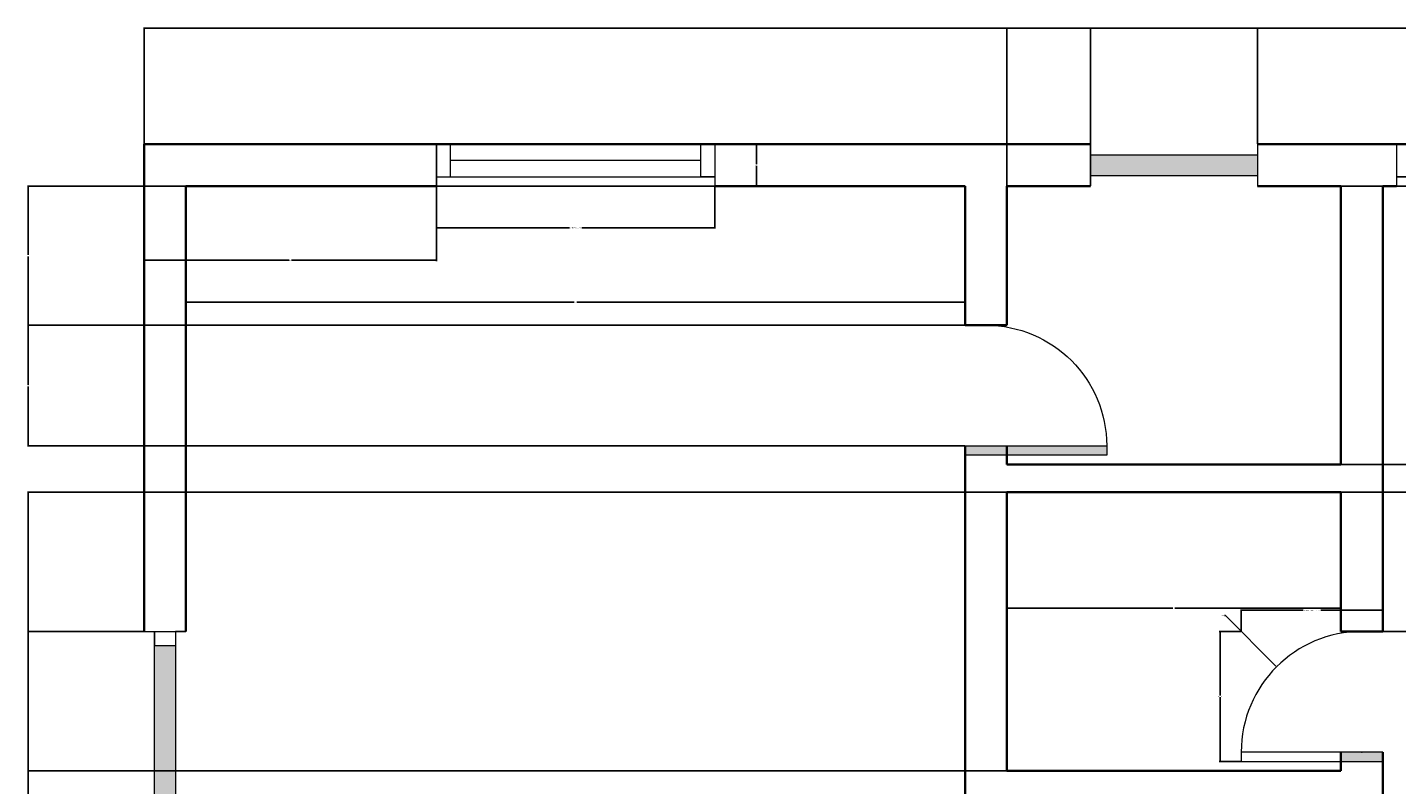
# Model space of a CAD drawing. Units: inches. Extents: x 2039 to 2485, y 1453 to 1986.
# Tile 3 of 4: x 2039 to 2334, y 1823 to 1986. Entities that reach past the tile are written whole.
import ezdxf

# ---------------------------------------------------------------- set-up
doc = ezdxf.new("R2010")
doc.units = ezdxf.units.IN
for name, color, linetype, lineweight in [('A-ANNO-DIMS', 2, 'Continuous', 18), ('A-DOOR', 3, 'Continuous', 18), ('A-GLAZ', 4, 'Continuous', 18), ('A-WALL', 7, 'Continuous', 35)]:
    doc.layers.add(name, color=color, linetype=linetype, lineweight=lineweight)
doc.layers.add('A-OPEN-PATT', color=18, linetype='Continuous', lineweight=13, true_color=0x000000)
doc.styles.get("Standard").update_dxf_attribs({"font": 'arial.ttf'})
doc.dimstyles.get("Standard").update_dxf_attribs({"dimtxt": 0.18, "dimasz": 0.18, "dimexe": 0.18, "dimexo": 0.0625, "dimgap": 0.09, "dimtad": 0, "dimtih": 1, "dimtoh": 1, "dimdec": 4, "dimzin": 0, "dimdsep": 46, "dimtxsty": 'Standard', "dimcen": 0.09, "dimadec": 0, "dimazin": 0, "dimtfac": 1, "dimtdec": 4, "dimtofl": 0, "dimtmove": 0, "dimatfit": 3, "dimfxl": 1, "dimtolj": 1, "dimtzin": 0, "dimarcsym": 0})

# ---------------------------------------------------------------- blocks, each defined once
blk = doc.blocks.new('DOOR-SWING-26IN')
for p, q in [((26, 2), (0, 2)), ((0, 2), (0, 0)), ((0, 0), (21.5, 0)), ((30.5, 2), (21.5, 2)), ((21.5, 0), (30.5, 0)), ((30.5, 0), (30.5, 2))]:
    blk.add_line(p, q)
blk.add_arc((26, 2), 26, 90, 180)
blk = doc.blocks.new('WIN-60IN')
for p, q in [((0, 0), (0, 9)), ((0, 9), (60, 9)), ((3, 2), (3, 9)), ((57, 2), (57, 9)), ((60, 9), (60, 0)), ((57, 5.5), (3, 5.5)), ((0, 2), (60, 2)), ((0, 0), (0, 2)), ((60, 2), (57, 2))]:
    blk.add_line(p, q)
blk = doc.blocks.new('*D8')
at = {"layer": 'A-ANNO-DIMS', "color": 0, "lineweight": -2, "transparency": 16777216}
for p, q in [((2300.5, 1856.12), (2300.5, 1860.81)), ((2300.68, 1860.63), (2313.86, 1860.63)), ((2330.82, 1860.63), (2317.65, 1860.63)), ((2331, 1856.12), (2331, 1860.81))]:
    blk.add_line(p, q, dxfattribs=at)
at = {"layer": 'A-ANNO-DIMS', "color": 0, "transparency": 16777216}
for points in [[(2300.68, 1860.66), (2300.68, 1860.6), (2300.5, 1860.63)], [(2330.82, 1860.66), (2330.82, 1860.6), (2331, 1860.63)]]:
    blk.add_solid(points, dxfattribs=at)
at = {"layer": 'Defpoints', "color": 0, "transparency": 16777216}
for p in [(2331, 1860.63), (2300.5, 1856.06), (2331, 1856.06)]:
    blk.add_point(p, dxfattribs=at)
at = {"layer": 'A-ANNO-DIMS', "color": 0, "transparency": 16777216, "insert": (2315.75, 1860.63), "char_height": 0.18, "attachment_point": 5}
blk.add_mtext('\\A1;D2 SWING ENVELOPE 31 TYP.', dxfattribs=at)
blk = doc.blocks.new('*D9')
at = {"layer": 'A-ANNO-DIMS', "color": 0, "lineweight": -2, "transparency": 16777216}
for p, q in [((2300.44, 1856.06), (2295.75, 1856.06)), ((2295.93, 1855.88), (2295.93, 1842.24)), ((2295.93, 1828.24), (2295.93, 1841.87)), ((2300.44, 1828.06), (2295.75, 1828.06))]:
    blk.add_line(p, q, dxfattribs=at)
at = {"layer": 'A-ANNO-DIMS', "color": 0, "transparency": 16777216}
for points in [[(2295.9, 1855.88), (2295.96, 1855.88), (2295.93, 1856.06)], [(2295.9, 1828.24), (2295.96, 1828.24), (2295.93, 1828.06)]]:
    blk.add_solid(points, dxfattribs=at)
at = {"layer": 'Defpoints', "color": 0, "transparency": 16777216}
for p in [(2295.93, 1856.06), (2300.5, 1856.06), (2300.5, 1828.06)]:
    blk.add_point(p, dxfattribs=at)
at = {"layer": 'A-ANNO-DIMS', "color": 0, "transparency": 16777216, "insert": (2295.93, 1842.06), "char_height": 0.18, "attachment_point": 5}
blk.add_mtext('\\A1;28 TYP.', dxfattribs=at)
blk = doc.blocks.new('*D10')
at = {"layer": 'A-ANNO-DIMS', "color": 0, "lineweight": -2, "transparency": 16777216}
for p, q in [((2127, 1951.99), (2127, 1942.88)), ((2187, 1951.99), (2187, 1942.88)), ((2127.18, 1943.06), (2155.66, 1943.06)), ((2186.82, 1943.06), (2158.34, 1943.06))]:
    blk.add_line(p, q, dxfattribs=at)
at = {"layer": 'A-ANNO-DIMS', "color": 0, "transparency": 16777216}
for points in [[(2127.18, 1943.09), (2127.18, 1943.03), (2127, 1943.06)], [(2186.82, 1943.09), (2186.82, 1943.03), (2187, 1943.06)]]:
    blk.add_solid(points, dxfattribs=at)
at = {"layer": 'Defpoints', "color": 0, "transparency": 16777216}
for p in [(2127, 1952.06), (2187, 1952.06), (2187, 1943.06)]:
    blk.add_point(p, dxfattribs=at)
at = {"layer": 'A-ANNO-DIMS', "color": 0, "transparency": 16777216, "insert": (2157, 1943.06), "char_height": 0.18, "attachment_point": 5}
blk.add_mtext('\\A1;WINDOW W1 60 TYP.', dxfattribs=at)
blk = doc.blocks.new('*D11')
at = {"layer": 'A-ANNO-DIMS', "color": 0, "lineweight": -2, "transparency": 16777216}
for p, q in [((2187.06, 1961.06), (2196.18, 1961.06)), ((2196, 1960.88), (2196, 1956.74)), ((2196, 1952.24), (2196, 1956.37)), ((2187.06, 1952.06), (2196.18, 1952.06))]:
    blk.add_line(p, q, dxfattribs=at)
at = {"layer": 'A-ANNO-DIMS', "color": 0, "transparency": 16777216}
for points in [[(2195.97, 1960.88), (2196.03, 1960.88), (2196, 1961.06)], [(2195.97, 1952.24), (2196.03, 1952.24), (2196, 1952.06)]]:
    blk.add_solid(points, dxfattribs=at)
at = {"layer": 'Defpoints', "color": 0, "transparency": 16777216}
for p in [(2187, 1961.06), (2196, 1961.06), (2187, 1952.06)]:
    blk.add_point(p, dxfattribs=at)
at = {"layer": 'A-ANNO-DIMS', "color": 0, "transparency": 16777216, "insert": (2196, 1956.56), "char_height": 0.18, "attachment_point": 5}
blk.add_mtext('\\A1;9 TYP.', dxfattribs=at)
blk = doc.blocks.new('*D16')
at = {"layer": 'A-ANNO-DIMS', "color": 0, "lineweight": -2, "transparency": 16777216}
for p, q in [((2064, 1961.12), (2064, 1986.25)), ((2064.18, 1986.07), (2261.71, 1986.07)), ((2459.82, 1986.07), (2262.29, 1986.07)), ((2460, 1961.12), (2460, 1986.25))]:
    blk.add_line(p, q, dxfattribs=at)
at = {"layer": 'A-ANNO-DIMS', "color": 0, "transparency": 16777216}
for points in [[(2064.18, 1986.1), (2064.18, 1986.04), (2064, 1986.07)], [(2459.82, 1986.1), (2459.82, 1986.04), (2460, 1986.07)]]:
    blk.add_solid(points, dxfattribs=at)
at = {"layer": 'Defpoints', "color": 0, "transparency": 16777216}
for p in [(2460, 1986.07), (2064, 1961.06), (2460, 1961.06)]:
    blk.add_point(p, dxfattribs=at)
at = {"layer": 'A-ANNO-DIMS', "color": 0, "transparency": 16777216, "insert": (2262, 1986.07), "char_height": 0.18, "attachment_point": 5}
blk.add_mtext('\\A1;396', dxfattribs=at)
blk = doc.blocks.new('*D18')
at = {"layer": 'A-ANNO-DIMS', "color": 0, "lineweight": -2, "transparency": 16777216}
for p, q in [((2064, 1960.99), (2064, 1935.87)), ((2127, 1960.99), (2127, 1935.87)), ((2064.18, 1936.05), (2095.28, 1936.05)), ((2126.82, 1936.05), (2095.72, 1936.05))]:
    blk.add_line(p, q, dxfattribs=at)
at = {"layer": 'A-ANNO-DIMS', "color": 0, "transparency": 16777216}
for points in [[(2064.18, 1936.08), (2064.18, 1936.02), (2064, 1936.05)], [(2126.82, 1936.08), (2126.82, 1936.02), (2127, 1936.05)]]:
    blk.add_solid(points, dxfattribs=at)
at = {"layer": 'Defpoints', "color": 0, "transparency": 16777216}
for p in [(2064, 1961.06), (2127, 1961.06), (2064, 1936.05)]:
    blk.add_point(p, dxfattribs=at)
at = {"layer": 'A-ANNO-DIMS', "color": 0, "transparency": 16777216, "insert": (2095.5, 1936.05), "char_height": 0.18, "attachment_point": 5}
blk.add_mtext('\\A1;63', dxfattribs=at)
blk = doc.blocks.new('*D28')
at = {"layer": 'A-ANNO-DIMS', "color": 0, "lineweight": -2, "transparency": 16777216}
for p, q in [((2063.94, 1856.06), (2038.81, 1856.06)), ((2038.99, 1855.88), (2038.99, 1826.24)), ((2038.99, 1796.24), (2038.99, 1825.87)), ((2063.94, 1796.06), (2038.81, 1796.06))]:
    blk.add_line(p, q, dxfattribs=at)
at = {"layer": 'A-ANNO-DIMS', "color": 0, "transparency": 16777216}
for points in [[(2038.96, 1855.88), (2039.02, 1855.88), (2038.99, 1856.06)], [(2038.96, 1796.24), (2039.02, 1796.24), (2038.99, 1796.06)]]:
    blk.add_solid(points, dxfattribs=at)
at = {"layer": 'Defpoints', "color": 0, "transparency": 16777216}
for p in [(2038.99, 1856.06), (2064, 1856.06), (2064, 1796.06)]:
    blk.add_point(p, dxfattribs=at)
at = {"layer": 'A-ANNO-DIMS', "color": 0, "transparency": 16777216, "insert": (2038.99, 1826.06), "char_height": 0.18, "attachment_point": 5}
blk.add_mtext('\\A1;60', dxfattribs=at)
blk = doc.blocks.new('*D38')
at = {"layer": 'A-ANNO-DIMS', "color": 0, "lineweight": -2, "transparency": 16777216}
for p, q in [((2073, 1951.99), (2073, 1926.87)), ((2241, 1951.99), (2241, 1926.87)), ((2073.18, 1927.05), (2156.72, 1927.05)), ((2240.82, 1927.05), (2157.28, 1927.05))]:
    blk.add_line(p, q, dxfattribs=at)
at = {"layer": 'A-ANNO-DIMS', "color": 0, "transparency": 16777216}
for points in [[(2073.18, 1927.08), (2073.18, 1927.02), (2073, 1927.05)], [(2240.82, 1927.08), (2240.82, 1927.02), (2241, 1927.05)]]:
    blk.add_solid(points, dxfattribs=at)
at = {"layer": 'Defpoints', "color": 0, "transparency": 16777216}
for p in [(2073, 1952.06), (2241, 1952.06), (2073, 1927.05)]:
    blk.add_point(p, dxfattribs=at)
at = {"layer": 'A-ANNO-DIMS', "color": 0, "transparency": 16777216, "insert": (2157, 1927.05), "char_height": 0.18, "attachment_point": 5}
blk.add_mtext('\\A1;168', dxfattribs=at)
blk = doc.blocks.new('*D43')
at = {"layer": 'A-ANNO-DIMS', "color": 0, "lineweight": -2, "transparency": 16777216}
for p, q in [((2250, 1885.99), (2250, 1860.87)), ((2322, 1885.99), (2322, 1860.87)), ((2250.18, 1861.05), (2285.79, 1861.05)), ((2321.82, 1861.05), (2286.22, 1861.05))]:
    blk.add_line(p, q, dxfattribs=at)
at = {"layer": 'A-ANNO-DIMS', "color": 0, "transparency": 16777216}
for points in [[(2250.18, 1861.08), (2250.18, 1861.02), (2250, 1861.05)], [(2321.82, 1861.08), (2321.82, 1861.02), (2322, 1861.05)]]:
    blk.add_solid(points, dxfattribs=at)
at = {"layer": 'Defpoints', "color": 0, "transparency": 16777216}
for p in [(2250, 1886.06), (2322, 1886.06), (2250, 1861.05)]:
    blk.add_point(p, dxfattribs=at)
at = {"layer": 'A-ANNO-DIMS', "color": 0, "transparency": 16777216, "insert": (2286, 1861.05), "char_height": 0.18, "attachment_point": 5}
blk.add_mtext('\\A1;72', dxfattribs=at)
blk = doc.blocks.new('*D44')
at = {"layer": 'A-ANNO-DIMS', "color": 0, "lineweight": -2, "transparency": 16777216}
for p, q in [((2250, 1952.12), (2250, 1986.25)), ((2250.18, 1986.07), (2258.79, 1986.07)), ((2267.82, 1986.07), (2259.21, 1986.07)), ((2268, 1952.12), (2268, 1986.25))]:
    blk.add_line(p, q, dxfattribs=at)
at = {"layer": 'A-ANNO-DIMS', "color": 0, "transparency": 16777216}
for points in [[(2250.18, 1986.1), (2250.18, 1986.04), (2250, 1986.07)], [(2267.82, 1986.1), (2267.82, 1986.04), (2268, 1986.07)]]:
    blk.add_solid(points, dxfattribs=at)
at = {"layer": 'Defpoints', "color": 0, "transparency": 16777216}
for p in [(2268, 1986.07), (2250, 1952.06), (2268, 1952.06)]:
    blk.add_point(p, dxfattribs=at)
at = {"layer": 'A-ANNO-DIMS', "color": 0, "transparency": 16777216, "insert": (2259, 1986.07), "char_height": 0.18, "attachment_point": 5}
blk.add_mtext('\\A1;18', dxfattribs=at)
blk = doc.blocks.new('*D45')
at = {"layer": 'A-ANNO-DIMS', "color": 0, "lineweight": -2, "transparency": 16777216}
for p, q in [((2268, 1961.12), (2268, 1986.25)), ((2268.18, 1986.07), (2285.78, 1986.07)), ((2303.82, 1986.07), (2286.22, 1986.07)), ((2304, 1961.12), (2304, 1986.25))]:
    blk.add_line(p, q, dxfattribs=at)
at = {"layer": 'A-ANNO-DIMS', "color": 0, "transparency": 16777216}
for points in [[(2268.18, 1986.1), (2268.18, 1986.04), (2268, 1986.07)], [(2303.82, 1986.1), (2303.82, 1986.04), (2304, 1986.07)]]:
    blk.add_solid(points, dxfattribs=at)
at = {"layer": 'Defpoints', "color": 0, "transparency": 16777216}
for p in [(2304, 1986.07), (2268, 1961.06), (2304, 1961.06)]:
    blk.add_point(p, dxfattribs=at)
at = {"layer": 'A-ANNO-DIMS', "color": 0, "transparency": 16777216, "insert": (2286, 1986.07), "char_height": 0.18, "attachment_point": 5}
blk.add_mtext('\\A1;36', dxfattribs=at)
blk = doc.blocks.new('*D46')
at = {"layer": 'A-ANNO-DIMS', "color": 0, "lineweight": -2, "transparency": 16777216}
for p, q in [((2322.06, 1952.06), (2485.19, 1952.06)), ((2485.01, 1951.88), (2485.01, 1922.24)), ((2485.01, 1892.24), (2485.01, 1921.87)), ((2322.06, 1892.06), (2485.19, 1892.06))]:
    blk.add_line(p, q, dxfattribs=at)
at = {"layer": 'A-ANNO-DIMS', "color": 0, "transparency": 16777216}
for points in [[(2484.98, 1951.88), (2485.04, 1951.88), (2485.01, 1952.06)], [(2484.98, 1892.24), (2485.04, 1892.24), (2485.01, 1892.06)]]:
    blk.add_solid(points, dxfattribs=at)
at = {"layer": 'Defpoints', "color": 0, "transparency": 16777216}
for p in [(2322, 1952.06), (2485.01, 1952.06), (2322, 1892.06)]:
    blk.add_point(p, dxfattribs=at)
at = {"layer": 'A-ANNO-DIMS', "color": 0, "transparency": 16777216, "insert": (2485.01, 1922.06), "char_height": 0.18, "attachment_point": 5}
blk.add_mtext('\\A1;60', dxfattribs=at)
blk = doc.blocks.new('*D47')
at = {"layer": 'A-ANNO-DIMS', "color": 0, "lineweight": -2, "transparency": 16777216}
for p, q in [((2249.94, 1886.06), (2038.81, 1886.06)), ((2038.99, 1885.88), (2038.99, 1856.24)), ((2038.99, 1826.24), (2038.99, 1855.87)), ((2249.94, 1826.06), (2038.81, 1826.06))]:
    blk.add_line(p, q, dxfattribs=at)
at = {"layer": 'A-ANNO-DIMS', "color": 0, "transparency": 16777216}
for points in [[(2038.96, 1885.88), (2039.02, 1885.88), (2038.99, 1886.06)], [(2038.96, 1826.24), (2039.02, 1826.24), (2038.99, 1826.06)]]:
    blk.add_solid(points, dxfattribs=at)
at = {"layer": 'Defpoints', "color": 0, "transparency": 16777216}
for p in [(2038.99, 1886.06), (2250, 1886.06), (2250, 1826.06)]:
    blk.add_point(p, dxfattribs=at)
at = {"layer": 'A-ANNO-DIMS', "color": 0, "transparency": 16777216, "insert": (2038.99, 1856.06), "char_height": 0.18, "attachment_point": 5}
blk.add_mtext('\\A1;60', dxfattribs=at)
blk = doc.blocks.new('*D49')
at = {"layer": 'A-ANNO-DIMS', "color": 0, "lineweight": -2, "transparency": 16777216}
for p, q in [((2249.94, 1826.06), (2038.81, 1826.06)), ((2038.99, 1825.88), (2038.99, 1823.24)), ((2038.99, 1820.24), (2038.99, 1822.87)), ((2249.94, 1820.06), (2038.81, 1820.06))]:
    blk.add_line(p, q, dxfattribs=at)
at = {"layer": 'A-ANNO-DIMS', "color": 0, "transparency": 16777216}
for points in [[(2038.96, 1825.88), (2039.02, 1825.88), (2038.99, 1826.06)], [(2038.96, 1820.24), (2039.02, 1820.24), (2038.99, 1820.06)]]:
    blk.add_solid(points, dxfattribs=at)
at = {"layer": 'Defpoints', "color": 0, "transparency": 16777216}
for p in [(2038.99, 1826.06), (2250, 1826.06), (2250, 1820.06)]:
    blk.add_point(p, dxfattribs=at)
at = {"layer": 'A-ANNO-DIMS', "color": 0, "transparency": 16777216, "insert": (2038.99, 1823.06), "char_height": 0.18, "attachment_point": 5}
blk.add_mtext('\\A1;6', dxfattribs=at)
blk = doc.blocks.new('*D50')
at = {"layer": 'A-ANNO-DIMS', "color": 0, "lineweight": -2, "transparency": 16777216}
for p, q in [((2322.06, 1892.06), (2485.19, 1892.06)), ((2485.01, 1891.88), (2485.01, 1889.24)), ((2485.01, 1886.24), (2485.01, 1888.87)), ((2322.06, 1886.06), (2485.19, 1886.06))]:
    blk.add_line(p, q, dxfattribs=at)
at = {"layer": 'A-ANNO-DIMS', "color": 0, "transparency": 16777216}
for points in [[(2484.98, 1891.88), (2485.04, 1891.88), (2485.01, 1892.06)], [(2484.98, 1886.24), (2485.04, 1886.24), (2485.01, 1886.06)]]:
    blk.add_solid(points, dxfattribs=at)
at = {"layer": 'Defpoints', "color": 0, "transparency": 16777216}
for p in [(2322, 1892.06), (2485.01, 1892.06), (2322, 1886.06)]:
    blk.add_point(p, dxfattribs=at)
at = {"layer": 'A-ANNO-DIMS', "color": 0, "transparency": 16777216, "insert": (2485.01, 1889.06), "char_height": 0.18, "attachment_point": 5}
blk.add_mtext('\\A1;6', dxfattribs=at)
blk = doc.blocks.new('*D51')
at = {"layer": 'A-ANNO-DIMS', "color": 0, "lineweight": -2, "transparency": 16777216}
for p, q in [((2240.94, 1952.06), (2038.81, 1952.06)), ((2038.99, 1951.88), (2038.99, 1937.24)), ((2038.99, 1922.24), (2038.99, 1936.87)), ((2240.94, 1922.06), (2038.81, 1922.06))]:
    blk.add_line(p, q, dxfattribs=at)
at = {"layer": 'A-ANNO-DIMS', "color": 0, "transparency": 16777216}
for points in [[(2038.96, 1951.88), (2039.02, 1951.88), (2038.99, 1952.06)], [(2038.96, 1922.24), (2039.02, 1922.24), (2038.99, 1922.06)]]:
    blk.add_solid(points, dxfattribs=at)
at = {"layer": 'Defpoints', "color": 0, "transparency": 16777216}
for p in [(2038.99, 1952.06), (2241, 1952.06), (2241, 1922.06)]:
    blk.add_point(p, dxfattribs=at)
at = {"layer": 'A-ANNO-DIMS', "color": 0, "transparency": 16777216, "insert": (2038.99, 1937.06), "char_height": 0.18, "attachment_point": 5}
blk.add_mtext('\\A1;30', dxfattribs=at)
blk = doc.blocks.new('*D52')
at = {"layer": 'A-ANNO-DIMS', "color": 0, "lineweight": -2, "transparency": 16777216}
for p, q in [((2240.94, 1922.06), (2038.81, 1922.06)), ((2038.99, 1921.88), (2038.99, 1909.24)), ((2038.99, 1896.24), (2038.99, 1908.87)), ((2240.94, 1896.06), (2038.81, 1896.06))]:
    blk.add_line(p, q, dxfattribs=at)
at = {"layer": 'A-ANNO-DIMS', "color": 0, "transparency": 16777216}
for points in [[(2038.96, 1921.88), (2039.02, 1921.88), (2038.99, 1922.06)], [(2038.96, 1896.24), (2039.02, 1896.24), (2038.99, 1896.06)]]:
    blk.add_solid(points, dxfattribs=at)
at = {"layer": 'Defpoints', "color": 0, "transparency": 16777216}
for p in [(2038.99, 1922.06), (2241, 1922.06), (2241, 1896.06)]:
    blk.add_point(p, dxfattribs=at)
at = {"layer": 'A-ANNO-DIMS', "color": 0, "transparency": 16777216, "insert": (2038.99, 1909.06), "char_height": 0.18, "attachment_point": 5}
blk.add_mtext('\\A1;26', dxfattribs=at)
blk = doc.blocks.new('*D53')
at = {"layer": 'A-ANNO-DIMS', "color": 0, "lineweight": -2, "transparency": 16777216}
for p, q in [((2322.06, 1886.06), (2485.19, 1886.06)), ((2485.01, 1885.88), (2485.01, 1871.24)), ((2485.01, 1856.24), (2485.01, 1870.87)), ((2331.06, 1856.06), (2485.19, 1856.06))]:
    blk.add_line(p, q, dxfattribs=at)
at = {"layer": 'A-ANNO-DIMS', "color": 0, "transparency": 16777216}
for points in [[(2484.98, 1885.88), (2485.04, 1885.88), (2485.01, 1886.06)], [(2484.98, 1856.24), (2485.04, 1856.24), (2485.01, 1856.06)]]:
    blk.add_solid(points, dxfattribs=at)
at = {"layer": 'Defpoints', "color": 0, "transparency": 16777216}
for p in [(2322, 1886.06), (2485.01, 1886.06), (2331, 1856.06)]:
    blk.add_point(p, dxfattribs=at)
at = {"layer": 'A-ANNO-DIMS', "color": 0, "transparency": 16777216, "insert": (2485.01, 1871.06), "char_height": 0.18, "attachment_point": 5}
blk.add_mtext('\\A1;30', dxfattribs=at)
blk = doc.blocks.new('*D68')
at = {"layer": 'A-ANNO-DIMS', "color": 0, "lineweight": -2, "transparency": 16777216}
for p, q in [((2296.91, 1859.47), (2297.09, 1859.47)), ((2297.09, 1859.47), (2307.99, 1848.57)), ((2326.41, 1830.06), (2326.59, 1830.06)), ((2326.5, 1829.97), (2326.5, 1830.15))]:
    blk.add_line(p, q, dxfattribs=at)
at = {"layer": 'A-ANNO-DIMS', "color": 0, "transparency": 16777216}
blk.add_solid([(2308.01, 1848.59), (2307.97, 1848.55), (2308.12, 1848.44)], dxfattribs=at)
at = {"layer": 'Defpoints', "color": 0, "transparency": 16777216}
for p in [(2308.12, 1848.44), (2326.5, 1830.06)]:
    blk.add_point(p, dxfattribs=at)
at = {"layer": 'A-ANNO-DIMS', "color": 0, "transparency": 16777216, "insert": (2296.41, 1859.47), "char_height": 0.18, "attachment_point": 5}
blk.add_mtext('\\A1;2X R26', dxfattribs=at)

msp = doc.modelspace()

# ---------------------------------------------------------------- hatches: boundary and pattern name
at = {"layer": 'A-OPEN-PATT'}
h = msp.add_hatch(color=256, dxfattribs=at)
h.dxf.hatch_style = 1
h.paths.add_polyline_path([(2070.75, 1853.06), (2066.25, 1853.06), (2066.25, 1799.06), (2070.75, 1799.06)])
h.paths.add_polyline_path([(2080, 1791.5, 0.013897), (2078, 1791.56), (2078, 1755.56), (2080, 1755.56)])
h.paths.add_polyline_path([(2070.75, 1712.06), (2066.25, 1712.06), (2066.25, 1670.06), (2070.75, 1670.06)])
h.paths.add_polyline_path([(2070.75, 1568.06), (2066.25, 1568.06), (2066.25, 1526.06), (2070.75, 1526.06)])
h.paths.add_polyline_path([(2080, 1518.5, 0.013897), (2078, 1518.56), (2078, 1482.56), (2080, 1482.56)])
h.paths.add_polyline_path([(2362.5, 1666.06), (2326.5, 1666.06), (2326.5, 1664.06), (2362.45, 1664.06, 0.013897)])
h.paths.add_polyline_path([(2457.75, 1601.06), (2453.25, 1601.06), (2453.25, 1553.06), (2457.75, 1553.06)])
h.paths.add_polyline_path([(2457.75, 1799.06), (2453.25, 1799.06), (2453.25, 1769.06), (2457.75, 1769.06)])
h.paths.add_polyline_path([(2336, 1791.5, 0.013897), (2334, 1791.56), (2334, 1755.56), (2336, 1755.56)])
h.paths.add_polyline_path([(2255, 1788.5, 0.015162), (2253, 1788.56), (2253, 1755.56), (2255, 1755.56)])
h.paths.add_polyline_path([(2331, 1830.06), (2322, 1830.06), (2322, 1828.06), (2331, 1828.06)])
h.paths.add_polyline_path([(2250, 1896.06), (2245.5, 1896.06), (2241, 1896.06), (2241, 1894.06), (2250, 1894.06)])
h.paths.add_polyline_path([(2271.5, 1896.06), (2250, 1896.06), (2250, 1894.06), (2271.5, 1894.06)])
h.paths.add_polyline_path([(2304, 1958.81), (2268, 1958.81), (2268, 1954.31), (2304, 1954.31)])

# ---------------------------------------------------------------- linework, layer by layer
at = {"layer": 'A-GLAZ'}
for p, q in [((2268, 1952.06), (2268, 1961.06)), ((2268, 1961.06), (2268, 1958.81)), ((2304, 1961.06), (2304, 1952.06)), ((2184, 1954.06), (2184, 1957.56)), ((2268, 1958.81), (2304, 1958.81)), ((2268, 1954.06), (2268, 1954.31)), ((2268, 1954.31), (2304, 1954.31)), ((2268, 1952.06), (2268, 1954.06)), ((2064, 1856.06), (2073, 1856.06)), ((2066.25, 1799.06), (2066.25, 1856.06)), ((2066.25, 1856.06), (2066.25, 1853.06)), ((2073, 1856.06), (2070.75, 1856.06)), ((2070.75, 1856.06), (2070.75, 1796.06)), ((2066.25, 1853.06), (2070.75, 1853.06))]:
    msp.add_line(p, q, dxfattribs=at)
at = {"layer": 'A-WALL'}
for p, q in [((2064, 1961.06), (2073, 1961.06)), ((2064, 1961.06), (2073, 1961.06)), ((2064, 1961.06), (2073, 1961.06)), ((2064, 1856.06), (2064, 1961.06)), ((2073, 1961.06), (2268, 1961.06)), ((2073, 1961.06), (2268, 1961.06)), ((2073, 1961.06), (2268, 1961.06)), ((2304, 1961.06), (2322, 1961.06)), ((2304, 1961.06), (2322, 1961.06)), ((2304, 1961.06), (2322, 1961.06)), ((2322, 1961.06), (2331, 1961.06)), ((2331, 1961.06), (2451, 1961.06)), ((2073, 1952.06), (2127, 1952.06)), ((2073, 1952.06), (2127, 1952.06)), ((2073, 1952.06), (2127, 1952.06)), ((2073, 1856.06), (2073, 1952.06)), ((2241, 1952.06), (2187, 1952.06)), ((2187, 1952.06), (2241, 1952.06)), ((2187, 1952.06), (2241, 1952.06)), ((2187, 1952.06), (2241, 1952.06)), ((2241, 1952.06), (2241, 1922.06)), ((2250, 1952.06), (2250, 1922.06)), ((2250, 1952.06), (2250, 1922.06)), ((2250, 1952.06), (2268, 1952.06)), ((2268, 1952.06), (2250, 1952.06)), ((2268, 1952.06), (2250, 1952.06)), ((2322, 1952.06), (2304, 1952.06)), ((2322, 1952.06), (2304, 1952.06)), ((2322, 1952.06), (2304, 1952.06)), ((2304, 1952.06), (2322, 1952.06)), ((2322, 1892.06), (2322, 1952.06)), ((2331, 1952.06), (2334, 1952.06)), ((2331, 1952.06), (2334, 1952.06)), ((2331, 1856.06), (2331, 1952.06)), ((2250, 1922.06), (2241, 1922.06)), ((2241, 1896.06), (2241, 1760.06)), ((2250, 1896.06), (2250, 1892.06)), ((2250, 1892.06), (2250, 1894.06)), ((2250, 1894.06), (2250, 1892.06)), ((2250, 1892.06), (2322, 1892.06)), ((2250, 1892.06), (2322, 1892.06)), ((2322, 1886.06), (2250, 1886.06)), ((2250, 1886.06), (2250, 1826.06)), ((2322, 1886.06), (2322, 1856.06)), ((2250, 1883.06), (2250, 1826.06)), ((2322, 1856.06), (2331, 1856.06)), ((2322, 1830.06), (2322, 1826.06)), ((2322, 1826.06), (2322, 1828.06)), ((2331, 1760.06), (2331, 1830.06)), ((2250, 1826.06), (2322, 1826.06))]:
    msp.add_line(p, q, dxfattribs=at)

# ---------------------------------------------------------------- block references
at = {"layer": 'A-DOOR', "extrusion": (0, 0, -1), "zscale": -1}
msp.add_blockref('DOOR-SWING-26IN', (-2271.5, 1894.06), dxfattribs=at)
at = {"layer": 'A-DOOR'}
msp.add_blockref('DOOR-SWING-26IN', (2300.5, 1828.06), dxfattribs=at)
at = {"layer": 'A-GLAZ'}
msp.add_blockref('WIN-60IN', (2127, 1952.06), dxfattribs=at)
at = {"layer": 'A-GLAZ', "extrusion": (0, 0, -1), "zscale": -1}
msp.add_blockref('WIN-60IN', (-2394, 1952.06), dxfattribs=at)

# ---------------------------------------------------------------- dimensions: what is measured, and where the dimension line sits
at = {"layer": 'A-ANNO-DIMS'}
for base, p1, p2, picture, middle in [((2460, 1986.07), (2064, 1961.06), (2460, 1961.06), '*D16', (2262, 1986.07)), ((2268, 1986.07), (2250, 1952.06), (2268, 1952.06), '*D44', (2259, 1986.07)), ((2304, 1986.07), (2268, 1961.06), (2304, 1961.06), '*D45', (2286, 1986.07))]:
    dim = msp.add_linear_dim(base=base, p1=p1, p2=p2, dimstyle='Standard', override={"dimdec": 0, "dimlfac": 1, "dimrnd": 0, "dimzin": 0, "dimdsep": 46, "dimlunit": 2}, dxfattribs=at)
    dim.commit()
    dim.dimension.update_dxf_attribs({"geometry": picture, "text_midpoint": middle})
for base, p1, p2, angle, picture, middle in [((2064, 1936.05), (2127, 1961.06), (2064, 1961.06), 180, '*D18', (2095.5, 1936.05)), ((2038.99, 1952.06), (2241, 1922.06), (2241, 1952.06), 90, '*D51', (2038.99, 1937.06)), ((2073, 1927.05), (2241, 1952.06), (2073, 1952.06), 180, '*D38', (2157, 1927.05)), ((2485.01, 1952.06), (2322, 1892.06), (2322, 1952.06), 90, '*D46', (2485.01, 1922.06)), ((2038.99, 1922.06), (2241, 1896.06), (2241, 1922.06), 90, '*D52', (2038.99, 1909.06)), ((2485.01, 1892.06), (2322, 1886.06), (2322, 1892.06), 90, '*D50', (2485.01, 1889.06)), ((2038.99, 1886.06), (2250, 1826.06), (2250, 1886.06), 90, '*D47', (2038.99, 1856.06)), ((2250, 1861.05), (2322, 1886.06), (2250, 1886.06), 180, '*D43', (2286, 1861.05)), ((2485.01, 1886.06), (2331, 1856.06), (2322, 1886.06), 90, '*D53', (2485.01, 1871.06)), ((2038.99, 1856.06), (2064, 1796.06), (2064, 1856.06), 90, '*D28', (2038.99, 1826.06)), ((2038.99, 1826.06), (2250, 1820.06), (2250, 1826.06), 90, '*D49', (2038.99, 1823.06))]:
    dim = msp.add_linear_dim(base=base, p1=p1, p2=p2, angle=angle, dimstyle='Standard', override={"dimdec": 0, "dimlfac": 1, "dimrnd": 0, "dimzin": 0, "dimdsep": 46, "dimlunit": 2}, dxfattribs=at)
    dim.commit()
    dim.dimension.update_dxf_attribs({"geometry": picture, "text_midpoint": middle})
for base, p1, p2, picture, middle in [((2196, 1961.06), (2187, 1952.06), (2187, 1961.06), '*D11', (2196, 1956.56)), ((2295.93, 1856.06), (2300.5, 1828.06), (2300.5, 1856.06), '*D9', (2295.93, 1842.06))]:
    dim = msp.add_linear_dim(base=base, p1=p1, p2=p2, angle=90, text='<> TYP.', dimstyle='Standard', override={"dimdec": 0, "dimlfac": 1, "dimrnd": 0, "dimzin": 0, "dimdsep": 46, "dimlunit": 2}, dxfattribs=at)
    dim.commit()
    dim.dimension.update_dxf_attribs({"geometry": picture, "text_midpoint": middle})
for base, p1, p2, text, picture, middle in [((2187, 1943.06), (2127, 1952.06), (2187, 1952.06), 'WINDOW W1 <> TYP.', '*D10', (2157, 1943.06)), ((2331.00241426, 1860.63110875), (2300.50241426, 1856.05610875), (2331.00241426, 1856.05610875), 'D2 SWING ENVELOPE <> TYP.', '*D8', (2315.75241426, 1860.63110875))]:
    dim = msp.add_linear_dim(base=base, p1=p1, p2=p2, text=text, dimstyle='Standard', override={"dimdec": 0, "dimlfac": 1, "dimrnd": 0, "dimzin": 0, "dimdsep": 46, "dimlunit": 2}, dxfattribs=at)
    dim.commit()
    dim.dimension.update_dxf_attribs({"geometry": picture, "text_midpoint": middle})
dim = msp.add_radius_dim(center=(2326.5, 1830.06), mpoint=(2308.12, 1848.44), text='2X <>', dimstyle='Standard', override={"dimdec": 0, "dimlfac": 1, "dimrnd": 0, "dimzin": 0, "dimdsep": 46, "dimlunit": 2}, dxfattribs=at)
dim.commit()
dim.dimension.update_dxf_attribs({"geometry": '*D68', "text_midpoint": (2296.41, 1859.47), "dimtype": 164})

doc.saveas('drawing.dxf')
